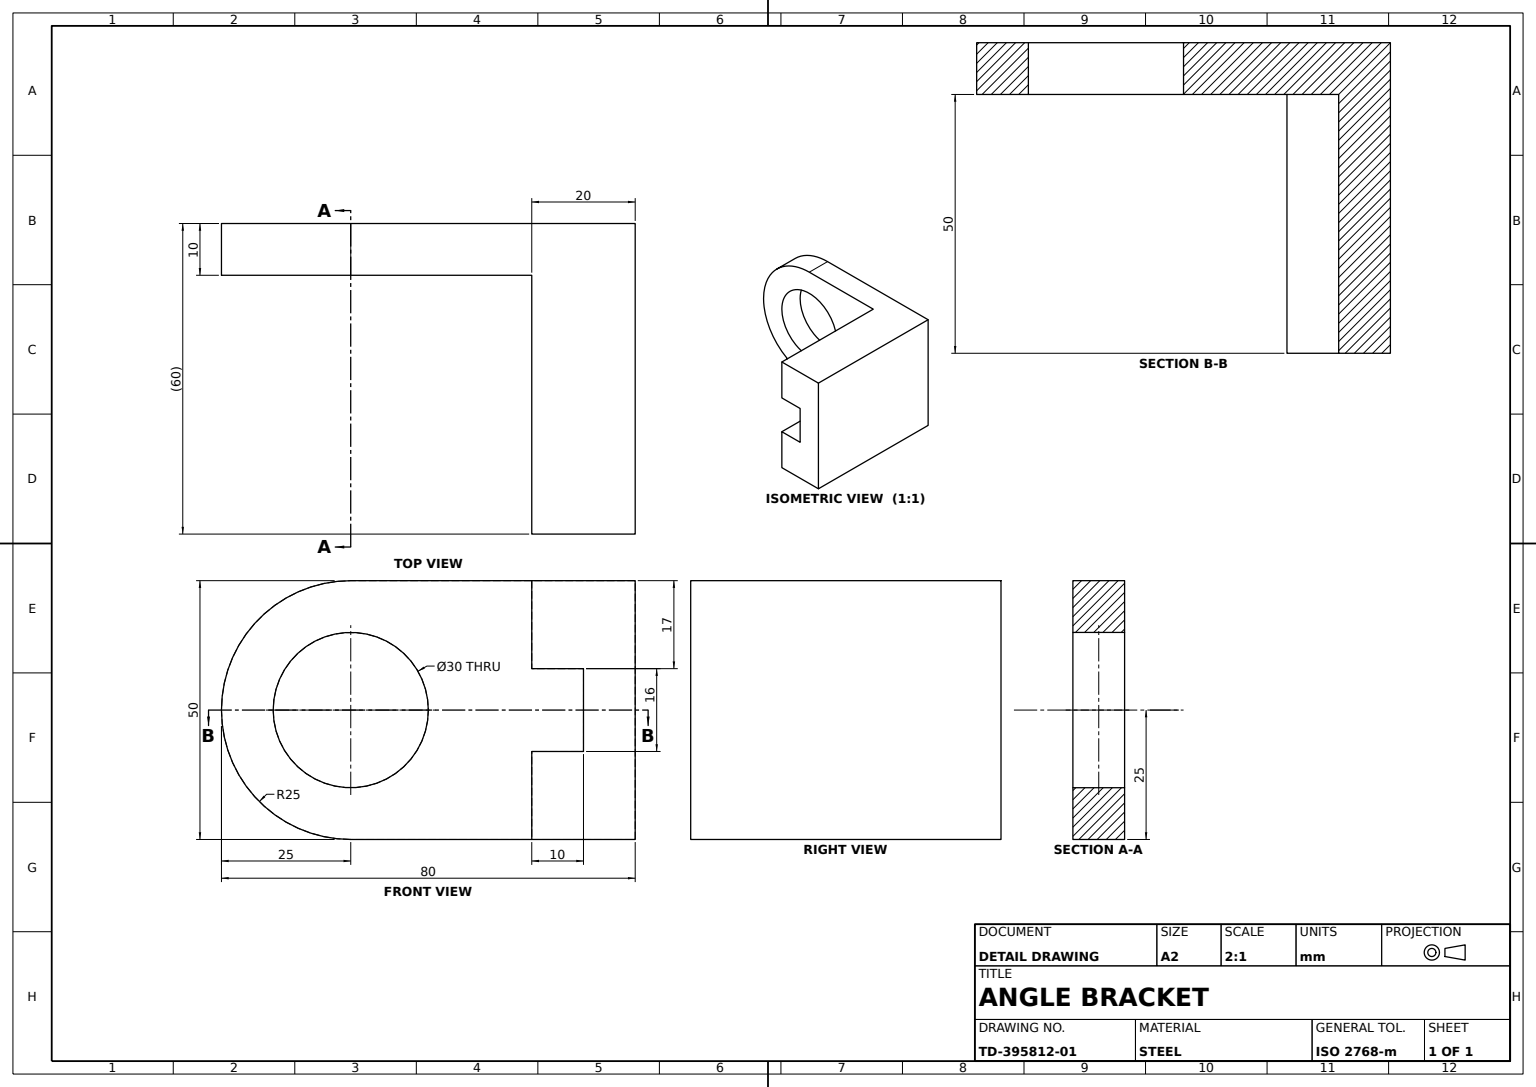
from build123d import *

# Parameters (mm, degrees)
BASE_PLATE_SKETCH_W    = 60
BASE_PLATE_SKETCH_H    = 50
BASE_PLATE_DEPTH       = 10
UPRIGHT_BLOCK_SKETCH_W = 10
UPRIGHT_BLOCK_SKETCH_H = 17
UPRIGHT_BLOCK_DEPTH    = 60
BLOCK_SLOT_SKETCH_W    = 10
BLOCK_SLOT_SKETCH_H    = 50
BLOCK_SLOT_DEPTH       = 10
ROUNDED_LUG_DEPTH      = 10
LUG_HOLE_SKETCH_R      = 15
LUG_HOLE_DEPTH         = 10


with BuildPart() as part:
    # Base Plate Sketch → Base Plate (new body)
    with BuildSketch(Plane.XY):
        with Locations((30, 25)):
            Rectangle(BASE_PLATE_SKETCH_W, BASE_PLATE_SKETCH_H)
    extrude(amount=BASE_PLATE_DEPTH)

    # Upright Block Sketch → Upright Block (add)
    with BuildSketch(Plane(origin=(60, 0, 0), x_dir=(0, 0, -1), z_dir=(1, 0, 0))):
        with Locations((-15, 41.5)):
            Rectangle(UPRIGHT_BLOCK_SKETCH_W, UPRIGHT_BLOCK_SKETCH_H)
        with Locations((-15, 8.5)):
            Rectangle(UPRIGHT_BLOCK_SKETCH_W, UPRIGHT_BLOCK_SKETCH_H)
    extrude(amount=-UPRIGHT_BLOCK_DEPTH)

    # Block Slot Sketch → Block Slot (cut)
    with BuildSketch(Plane.XY.offset(20)):
        with Locations((5, 25)):
            Rectangle(BLOCK_SLOT_SKETCH_W, BLOCK_SLOT_SKETCH_H)
    extrude(amount=-BLOCK_SLOT_DEPTH, mode=Mode.SUBTRACT)

    # Rounded Lug Sketch → Rounded Lug (add)
    with BuildSketch(Plane.ZY):
        with BuildLine():
            Line((20, 50), (10, 50))
            Line((10, 50), (10, 0))
            Line((10, 0), (20, 0))
            Line((20, 0), (55, 0))
            ThreePointArc((55, 0), (80, 25), (55, 50))
            Line((55, 50), (20, 50))
        make_face()
    extrude(amount=-ROUNDED_LUG_DEPTH)

    # Lug Hole Sketch → Lug Hole (cut)
    with BuildSketch(Plane(origin=(10, 0, 0), x_dir=(0, 0, -1), z_dir=(1, 0, 0))):
        with Locations((-55, 25)):
            Circle(LUG_HOLE_SKETCH_R)
    extrude(amount=-LUG_HOLE_DEPTH, mode=Mode.SUBTRACT)


solid = part.part
